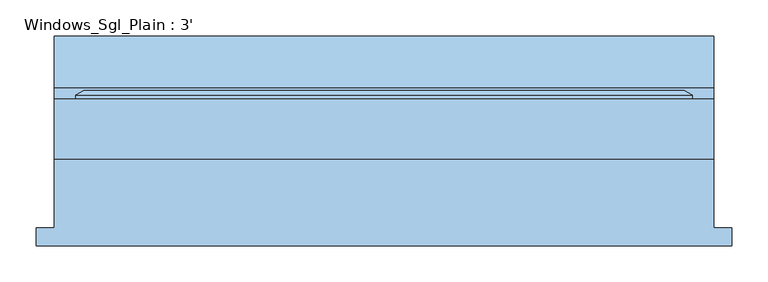
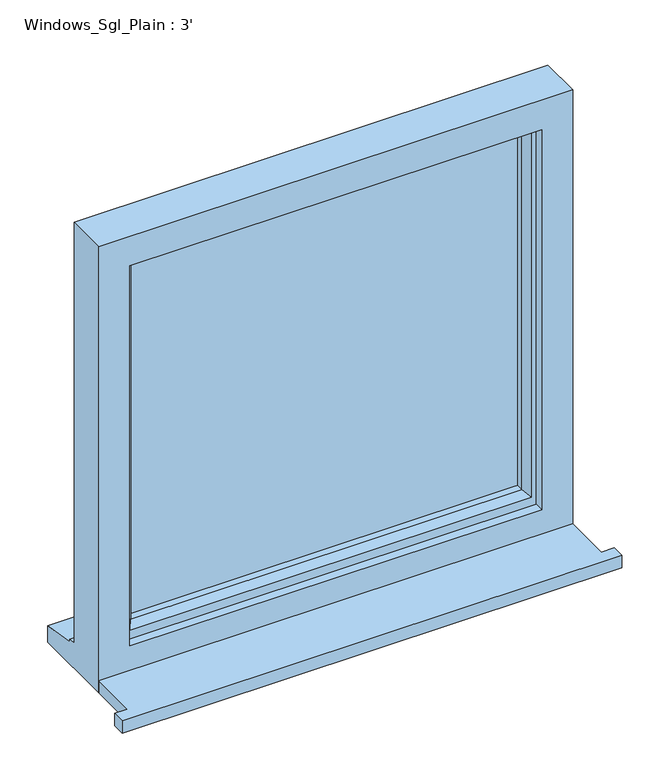
"""IFC4 building model written with IfcOpenShell, lengths in millimetres: window geometry, Windows_Sgl_Plain : 3'."""

from ifc_helpers import new_model, si_unit, frame, origin, place, context, project, spatial, polyline, outline, extrude, faceted_brep, source, transform, mapped, element, save


def windows_sgl_plain_3_28d0678b(model_context):
    return source(origin(), model_context, "Body", "SolidModel", [
        extrude(outline(polyline([(-482.2, -130.8434322), (-482.2, -105.8434322), (-457.2, -105.8434322), (-457.2, -10.2434322), (457.2, -10.2434322), (457.2, -105.8434322), (482.2, -105.8434322), (482.2, -130.8434322), (-482.2, -130.8434322)])), frame((0.0, 0.0, 1200.0), z_axis=(0.0, 0.0, 1.0), x_axis=(1.0, 0.0, 0.0)), (0.0, 0.0, 1.0), 25.0),
        faceted_brep([(-457.2, -10.2434322, 1200.0), (457.2, -10.2434322, 1200.0), (457.2, -10.2434322, 2110.0), (-457.2, -10.2434322, 2110.0), (-397.2, -10.2434322, 2050.0), (397.2, -10.2434322, 2050.0), (397.2, -10.2434322, 1275.0), (-397.2, -10.2434322, 1275.0), (-457.2, 72.7565678, 2110.0), (-457.2, 72.7565678, 1251.0), (-457.2, 87.7565678, 1249.68767), (-457.2, 87.7565678, 1244.7449676), (-457.2, 160.2565678, 1233.8088847), (-457.2, 160.2565678, 1200.0), (457.2, 72.7565678, 2110.0), (457.2, 72.7565678, 1251.0), (-417.2, 72.7565678, 2070.0), (-417.2, 72.7565678, 1263.0), (417.2, 72.7565678, 1263.0), (417.2, 72.7565678, 2070.0), (-417.2, 7.7565678, 2070.0), (-417.2, 7.7565678, 1263.0), (417.2, 7.7565678, 2070.0), (417.2, 7.7565678, 1263.0), (-397.2, 7.7565678, 2050.0), (-397.2, 7.7565678, 1275.0), (397.2, 7.7565678, 1275.0), (397.2, 7.7565678, 2050.0), (457.2, 160.2565678, 1200.0), (457.2, 160.2565678, 1233.8088847), (457.2, 87.7565678, 1244.7449676), (457.2, 87.7565678, 1249.68767)], [[[0, 1, 2, 3], [4, 5, 6, 7]], [[0, 3, 8, 9, 10, 11, 12, 13]], [[9, 8, 14, 15], [16, 17, 18, 19]], [[17, 16, 20, 21]], [[20, 22, 23, 21], [24, 25, 26, 27]], [[24, 4, 7, 25]], [[3, 2, 14, 8]], [[16, 19, 22, 20]], [[5, 4, 24, 27]], [[15, 14, 2, 1, 28, 29, 30, 31]], [[19, 18, 23, 22]], [[5, 27, 26, 6]], [[28, 1, 0, 13]], [[29, 28, 13, 12]], [[30, 29, 12, 11]], [[31, 30, 11, 10]], [[15, 31, 10, 9]], [[21, 23, 18, 17]], [[7, 6, 26, 25]]]),
        extrude(outline(polyline([(387.2, 36.7565678), (-387.2, 36.7565678), (-387.2, 60.7565678), (387.2, 60.7565678), (387.2, 36.7565678)])), frame((0.0, 0.0, 1293.0), z_axis=(0.0, 0.0, 1.0), x_axis=(1.0, 0.0, 0.0)), (0.0, 0.0, 1.0), 747.0),
        faceted_brep([(-427.2, 72.7565678, 2080.0), (-427.2, 78.5300705, 2080.0), (-427.2, 78.5300705, 1253.0), (-427.2, 72.7565678, 1253.0), (-417.2, 7.7565678, 2070.0), (-417.2, 72.7565678, 2070.0), (-417.2, 72.7565678, 1263.0), (-417.2, 7.7565678, 1263.0), (-377.2, 22.2494677, 2030.0), (-387.3480377, 7.7565678, 2040.1480377), (-387.3480377, 7.7565678, 1292.8519623), (-377.2, 22.2494677, 1303.0), (-377.2, 36.7565678, 2030.0), (-377.2, 36.7565678, 1303.0), (-387.2, 60.7565678, 2040.0), (-387.2, 36.7565678, 2040.0), (-387.2, 36.7565678, 1293.0), (-387.2, 60.7565678, 1293.0), (-377.2, 78.5300705, 2030.0), (-377.2, 60.7565678, 2030.0), (-377.2, 60.7565678, 1303.0), (-377.2, 78.5300705, 1303.0), (-394.6457548, 84.3035732, 2047.4457548), (-394.6457548, 84.3035732, 1285.5542452), (-416.4153903, 84.3035732, 2069.2153903), (-416.4153903, 84.3035732, 1263.7846097), (427.2, 78.5300705, 1253.0), (427.2, 72.7565678, 1253.0), (417.2, 72.7565678, 1263.0), (417.2, 7.7565678, 1263.0), (387.3480377, 7.7565678, 1292.8519623), (377.2, 22.2494677, 1303.0), (377.2, 36.7565678, 1303.0), (387.2, 36.7565678, 1293.0), (387.2, 60.7565678, 1293.0), (377.2, 60.7565678, 1303.0), (377.2, 78.5300705, 1303.0), (394.6457548, 84.3035732, 1285.5542452), (416.4153903, 84.3035732, 1263.7846097), (427.2, 78.5300705, 2080.0), (427.2, 72.7565678, 2080.0), (417.2, 72.7565678, 2070.0), (417.2, 7.7565678, 2070.0), (387.3480377, 7.7565678, 2040.1480377), (377.2, 22.2494677, 2030.0), (377.2, 36.7565678, 2030.0), (387.2, 36.7565678, 2040.0), (387.2, 60.7565678, 2040.0), (377.2, 60.7565678, 2030.0), (377.2, 78.5300705, 2030.0), (394.6457548, 84.3035732, 2047.4457548), (416.4153903, 84.3035732, 2069.2153903)], [[[0, 1, 2, 3]], [[4, 5, 6, 7]], [[8, 9, 10, 11]], [[12, 8, 11, 13]], [[14, 15, 16, 17]], [[18, 19, 20, 21]], [[22, 18, 21, 23]], [[1, 24, 25, 2]], [[3, 2, 26, 27]], [[7, 6, 28, 29]], [[11, 10, 30, 31]], [[13, 11, 31, 32]], [[17, 16, 33, 34]], [[21, 20, 35, 36]], [[23, 21, 36, 37]], [[2, 25, 38, 26]], [[27, 26, 39, 40]], [[29, 28, 41, 42]], [[31, 30, 43, 44]], [[32, 31, 44, 45]], [[34, 33, 46, 47]], [[36, 35, 48, 49]], [[37, 36, 49, 50]], [[26, 38, 51, 39]], [[40, 39, 1, 0]], [[3, 27, 40, 0], [5, 41, 28, 6]], [[42, 41, 5, 4]], [[7, 29, 42, 4], [9, 43, 30, 10]], [[44, 43, 9, 8]], [[45, 44, 8, 12]], [[15, 46, 33, 16], [13, 32, 45, 12]], [[47, 46, 15, 14]], [[17, 34, 47, 14], [19, 48, 35, 20]], [[49, 48, 19, 18]], [[50, 49, 18, 22]], [[24, 51, 38, 25], [23, 37, 50, 22]], [[39, 51, 24, 1]]]),
    ])


if __name__ == "__main__":
    model = new_model("IFC4")
    model_context = context("Model", 3, world=origin())
    ifc_project = project(units=[si_unit("LENGTHUNIT", "METRE", prefix="MILLI")], contexts=[model_context])
    site = spatial("IfcSite", under=ifc_project)
    building = spatial("IfcBuilding", under=site)
    placement = place(None, origin())
    windows_sgl_plain_3_shape = windows_sgl_plain_3_28d0678b(model_context)
    element("IfcWindow", 1, ObjectType="Windows_Sgl_Plain : 3'", at=placement, inside=building, context=model_context, shape_type="MappedRepresentation", body=[
        mapped(windows_sgl_plain_3_shape, transform((0.0, 0.0, 0.0), x_axis=(1.0, 0.0, 0.0), y_axis=(0.0, 1.0, 0.0), z_axis=(0.0, 0.0, 1.0))),
    ])
    save(model, "model.ifc")

# Revit data of these elements
# Type "Windows_Sgl_Plain : 3'"
#   Type Mark = "66"
#   Operation = "SinglePanel"
#   Construction Type Id = "SGL"
#   Manufacturer = "Revit"
#   Keynote = "L10"
#   Analytic Construction = "Large single-glazed windows"
#   Wrap Layers (Ext) from Ext = 0' - 4.03543"
#   Wrap Layers (Int) from Ext = 0' - 6.98819"
#   Window Board Projection = 0' - 0.98425"
#   Window Board Extension = 0' - 0.98425"
#   Visual Light Transmittance = 0.9
#   Solar Heat Gain Coefficient = 0.86
#   Rough Width = 3' - 0"
#   Rough Height = 2' - 11.82677"
#   Height = 2' - 11.82677"
#   Width = 3' - 0"
#   Heat Transfer Coefficient (U) = 5.5617 W/(m²·K)
#   Glazing Thickness = 0' - 0.94488"
#   FrameOffset - External = 0' - 1.9685"
#   Frame Depth = 0' - 2.55906"
#   Default Head Height = 6' - 11.07087"
#   Cill Depth = 0' - 3.44488"
#   Cavity Closer Width = 0' - 1.9685"
#   Cavity Closer Offset from Ext = 0' - 4.03543"
#   Cavity Closer Depth = 0' - 3.34646"
#   Vis - Cavity Closers = yes
#   Define Thermal Properties by = 1
#   Material Trim = Window Frame
#   Material Glass = Glass
#   Material Frame = Window Frame
#   Wall Closure = (empty or 0)
# Element 1 (IfcWindow, "Windows_Sgl_Plain : 3'")
#   Materials on its faces: "Window Frame", "Glass"
# Materials
#   "Window Frame": colour RGB 249 249 249, transparency 0, Keynote = "L10", Cost = 0
#   "Glass": class "Glass", colour RGB 0 128 192, transparency 0.9, Description = "Soda Lime Glass", Cost = 0
